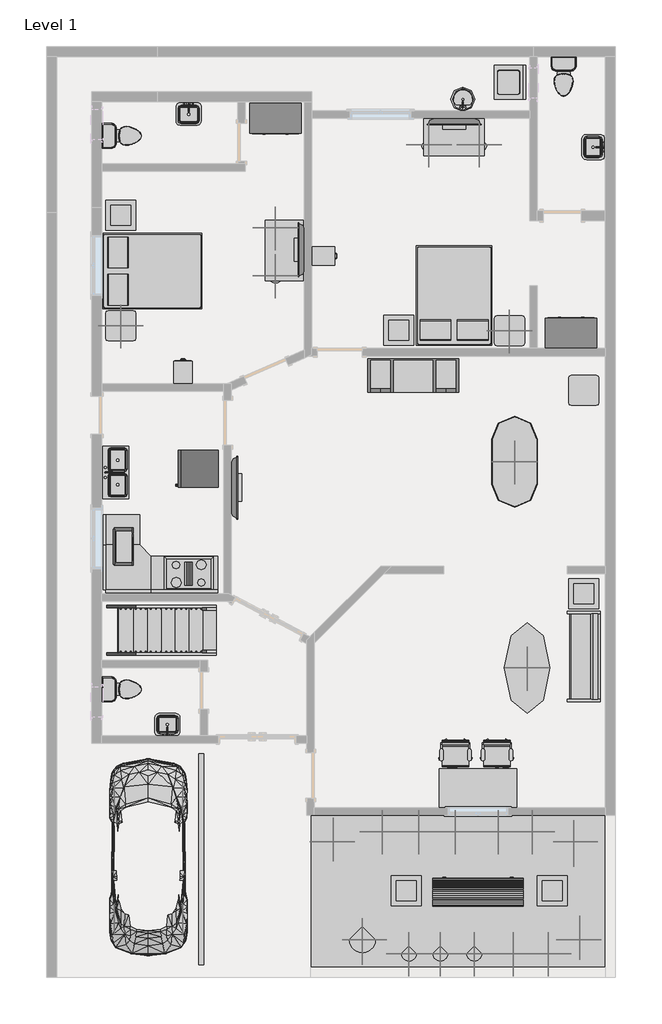
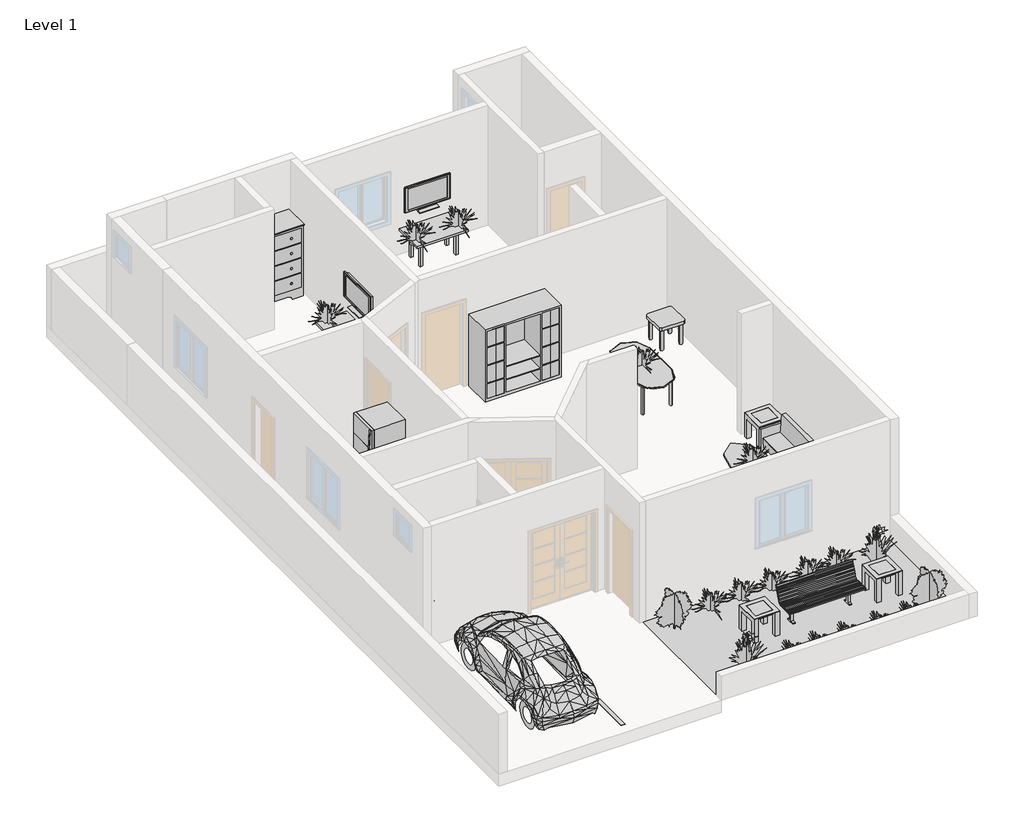
# One storey, part 2 of 2: 27 furniture elements, 23 geographic elements, 12 flow terminals, 7 proxies, 2 members, 2 railings, 1 stair flight.
# Revit data of these elements (continued)
# Type "RPC Plant - Tropical : Jungle Flame - 3'" (continued)
#   built-in parameter 1005198 = "{2, 15},{39, RPC-16-FUVJ-JWG0-MWGK-8000-ST1L-LVER-AU},{1, 0},{1, 0},{2, 13},{1, 8},{5, Color},{1, 0},{1, 0},{3, 0.8},{3, 0.8},{3, 0.8},{1, 8},{7, BBoxMin},{1, 0},{1, 0},{1, 0},{1, 0},{1, 0},{1, 8},{7, BBoxMax},{1, 0},{1, 0},{1, 0},{1, 0},{1, 0},{2, 11},{9, RPCTypeId},{1, 0},{1, 0},{39, RPC-16-FUVJ-JWG0-MWGK-8000-ST1L-LVER-AU},{1, 6},{14, RPCPlantHeight},{1, 0},{1, 0},{1, 3},{2, 11},{7, keyword},{1, 0},{1, 0},{35, :RPCs:Shrubs [General]:Geometry:RPC},{2, 11},{8, category},{1, 0},{1, 0},{16, Shrubs [General]},{2, 11},{12, LocalizedUID},{1, 0},{1, 0},{12, Jungle Flame},{2, 14},{6, Height},{1, 0},{1, 0},{1, 3},{1, 2},{16, Cast Reflections},{1, 0},{1, 0},{1, 0},{1, 2},{12, Cast Shadows},{1, 0},{1, 0},{1, 1},{1, 2},{9, Lock View},{1, 0},{1, 0},{1, 0},{1, 4},{5, ViewC},{1, 0},{1, 0},{1, 0},{21, assetlibrary_base.fbx},{1, 5},"
#   built-in parameter 1005195 = "RPC-16-FUVJ-JWG0-MWGK-8000-ST1L-LVER-AU"
#   Type Comments = "Jungle Flame"
#   Assembly Code = "G2050500"
#   Height = 3' - 0"
#   Default Elevation = 0
# Type "Handrail - Rectangular"
#   Assembly Code = "C2010400"
#   built-in parameter 1008612 = 0.0416667 (stored number, unit not read)
#   built-in parameter 1008611 = 0.0416667 (stored number, unit not read)
#   built-in parameter 1008609 = 0.333333 (stored number, unit not read)
#   built-in parameter 1008604 = 0.166667 (stored number, unit not read)
#   built-in parameter 1008603 = 0.166667 (stored number, unit not read)
#   Railing Height = 3' - 0"
#   built-in parameter 1008630 = 2
#   built-in parameter 1008610 = 2
#   built-in parameter 1008618 = Baluster - Square : 3/4"
# Element 1 (IfcBuildingElementProxy)
#   Material = Plant
#   Phase Created = New Construction
# Element 2 (IfcBuildingElementProxy, "Cook Top-4 Unit : 36\" x 20\"")
#   Phase Created = New Construction
#   Materials on its faces: "Steel, Chrome Plated", "Steel, Polished"
# Element 3 (IfcBuildingElementProxy, "Microwave : 30\" x 16\" x 18\"")
#   Phase Created = New Construction
#   Materials on its faces: "Laminate, Linen, Matte", "Glass"
# Element 4 (IfcBuildingElementProxy, "Parking Space : 9' x 18' - 90 deg")
#   Phase Created = New Construction
#   Materials on its faces: "Parking Stripe"
# Element 5 (IfcBuildingElementProxy, "RPC Beetle : RPC Beetle")
#   Phase Created = New Construction
# Element 6 (IfcBuildingElementProxy, "Refrigerator : 30\" x 32\" RH")
#   Phase Created = New Construction
#   Materials on its faces: "Steel, Paint Finish, Ivory, Glossy", "Steel, Chrome Plated"
# Element 7 (IfcBuildingElementProxy, "Washer : 27\" x 25\" x 35\"")
#   Phase Created = New Construction
#   Materials on its faces: "Steel, Paint Finish, Ivory, Matte"
# Element 8 (IfcFlowTerminal, "Floor Drain - Round : 5\" Strainer - 2\" Drain")
#   Mark = "3"
#   Phase Created = New Construction
# Element 9 (IfcFlowTerminal, "Floor Drain - Round : 5\" Strainer - 2\" Drain")
#   Mark = "7"
#   Phase Created = New Construction
# Element 10 (IfcFlowTerminal, "Floor Drain - Round : 5\" Strainer - 2\" Drain")
#   Mark = "14"
#   Phase Created = New Construction
# Element 11 (IfcFlowTerminal, "Floor Drain - Round : 5\" Strainer - 2\" Drain")
#   Mark = "16"
#   Phase Created = New Construction
# Element 12 (IfcFlowTerminal, "Sink Kitchen-Double : 42\" x 21\"")
#   Mark = "11"
#   Phase Created = New Construction
#   Materials on its faces: "Steel, Polished"
# Element 13 (IfcFlowTerminal, "Sink Vanity-Round : 19\" x 19\"")
#   Mark = "15"
#   Phase Created = New Construction
#   Materials on its faces: "Porcelain, Linen", "Steel, Polished"
# Element 14 (IfcFlowTerminal, "Sink Vanity-Square : 20\" x 18\"")
#   Mark = "4"
#   Phase Created = New Construction
#   Materials on its faces: "Porcelain, Linen", "Steel, Polished"
# Element 15 (IfcFlowTerminal, "Sink Vanity-Square : 20\" x 18\"")
#   Mark = "8"
#   Phase Created = New Construction
#   Materials on its faces: "Porcelain, Linen", "Steel, Polished"
# Element 16 (IfcFlowTerminal, "Sink Vanity-Square : 20\" x 18\"")
#   Mark = "13"
#   Phase Created = New Construction
#   Materials on its faces: "Porcelain, Linen", "Steel, Polished"
# Element 17 (IfcFlowTerminal, "Toilet-Domestic-3D : Toilet-Domestic-3D")
#   Mark = "6"
#   Phase Created = New Construction
#   Materials on its faces: "Porcelain, Linen", "Laminate, Linen, Matte"
# Element 18 (IfcFlowTerminal, "Toilet-Domestic-3D : Toilet-Domestic-3D")
#   Mark = "10"
#   Phase Created = New Construction
#   Materials on its faces: "Porcelain, Linen", "Laminate, Linen, Matte"
# Element 19 (IfcFlowTerminal, "Toilet-Domestic-3D : Toilet-Domestic-3D")
#   Mark = "12"
#   Phase Created = New Construction
#   Materials on its faces: "Porcelain, Linen", "Laminate, Linen, Matte"
# Elements 20, 21 (IfcFurniture, "Bed-Box : Queen 60\" x 79\"")
#   Phase Created = New Construction
#   Materials on its faces: "Birch", "Sash"
# Elements 22, 23 (IfcFurniture, "Cabinet-File 2 Drawer : 15\" x 18\"")
#   Phase Created = New Construction
#   Materials on its faces: "Steel, Chrome Plated", "Steel, Paint Finish, Ivory, Glossy"
# Elements 24, 25 (IfcFurniture, "Chair-Task Arms : Chair-Task Arms")
#   Phase Created = New Construction
#   Materials on its faces: "Plastic, Opaque Black", "Textile - Slate Blue"
# Element 26 (IfcFurniture, "Desk : 60\" x 30\" Student")
#   Phase Created = New Construction
#   Materials on its faces: "Steel, Chrome Plated", "Laminate, Ivory, Matte", "Cherry"
# Elements 27, 28 (IfcFurniture, "Dresser : 48\" x 72\" x 24\"")
#   Phase Created = New Construction
#   Materials on its faces: "Laminate, Ivory, Matte", "Cherry", "Wood"
# Element 29 (IfcFurniture, "Entertainment Center : 72\" x 72\" x 24\"")
#   Phase Created = New Construction
#   Materials on its faces: "Wood - Teak", "Steel, Chrome Plated", "Glass - Clear, Grey"
# Element 30 (IfcFurniture, "Sofa : 72\"")
#   Phase Created = New Construction
#   Materials on its faces: "Cherry", "Linen, Beige"
# Elements 31, 32 (IfcFurniture, "TV - Flat Screen : 42\"")
#   Stand = yes
#   Phase Created = New Construction
#   Materials on its faces: "TV - Black", "TV - Glass", "TV - Screen"
# Element 33 (IfcFurniture, "TV - Flat Screen : 50\"")
#   Stand = yes
#   Phase Created = New Construction
#   Materials on its faces: "TV - Black", "TV - Glass", "TV - Screen"
# Elements 34, 35, 36, 37, 38 (IfcFurniture, "Table-Coffee : 24\" x 24\" x 24\"")
#   Phase Created = New Construction
#   Materials on its faces: "Glass - Clear, Grey"
# Element 39 (IfcFurniture, "Table-Dining Oval : 36\" x 72\"")
#   Phase Created = New Construction
#   Materials on its faces: "Steel, Chrome Plated", "Glass - Clear, Grey"
# Element 40 (IfcFurniture, "Table-Ellipse : 72\" x 36\"")
#   Phase Created = New Construction
#   Materials on its faces: "Birch", "Plywood, Sheathing"
# Elements 41, 42, 43 (IfcFurniture, "Table-End : 24\" x 24\"")
#   Phase Created = New Construction
#   Materials on its faces: "Laminate, Ivory, Matte", "Birch"
# Elements 44, 45 (IfcFurniture, "Table-Rectangular : 72\" x 30\"")
#   Phase Created = New Construction
#   Materials on its faces: "Birch"
# Element 46 (IfcFurniture, "Work Station Cubicle : 96\" x 96\"")
#   Phase Created = New Construction
#   Materials on its faces: "Textile - Light Gray", "Laminate, Ivory, Matte"
# Element 47 (IfcGeographicElement, "Park Bench : 72\"")
#   Phase Created = New Construction
#   Materials on its faces: "Wood - Teak", "Steel, Paint Finish, Dark Gray, Matte"
# Elements 48, 49 (IfcGeographicElement, "RPC Plant - Tropical")
#   Phase Created = New Construction
# Elements 50, 51, 52, 53, 54, 55, 56, 57, 58, 59, 60, 61, 62, 63, 64, 65, 66, 67 (IfcGeographicElement, "RPC Plant - Tropical : Agave - 1.5'")
#   Phase Created = New Construction
# Elements 68, 69 (IfcGeographicElement, "RPC Plant - Tropical : Jungle Flame - 3'")
#   Phase Created = New Construction
# Elements 70, 71 (IfcMember, "Stringer - 2\" Width")
#   Phase Created = New Construction
# Elements 72, 73 (IfcRailing, "Handrail - Rectangular")
#   Phase Created = New Construction
# Element 74 (IfcStairFlight, "2\" Tread 1\" Nosing 1/4\" Riser")
#   Phase Created = New Construction
# Materials
#   "Steel, Chrome Plated": class "Metal", colour RGB 17 17 17, transparency 0, Description = "Chromiuim plated steel", Cost = 0
#   "Steel, Polished": class "Metal", colour RGB 57 57 57, transparency 0, Description = "Polished steel", Cost = 0
#   "Laminate, Linen, Matte": class "Plastic", colour RGB 249 239 230, transparency 0, Description = "Plastic Laminate - Linen, Matte", Cost = 0
#   "Steel, Paint Finish, Ivory, Glossy": class "Metal", colour RGB 247 247 239, transparency 0, Description = "Steel, paint finish, ivory, glossy", Cost = 0
#   "Steel, Paint Finish, Ivory, Matte": class "Metal", colour RGB 247 247 239, transparency 0, Description = "Steel, paint finish, ivory, matte", Cost = 0
#   "Porcelain, Linen": class "Ceramic", colour RGB 249 239 230, transparency 0, Description = "Porcelain, linen", Cost = 0
#   "Birch": class "Wood", colour RGB 210 159 95, transparency 0, Description = "Betula Alleghaniensis", Cost = 0
#   "Sash": class "Wood", colour RGB 224 178 126, transparency 0
#   "Plastic, Opaque Black": class "Plastic", colour RGB 0 0 0, transparency 0.7, Description = "Plastic, generic, opaque black", Cost = 0
#   "Textile - Slate Blue": class "Fabric", colour RGB 98 102 118, transparency 0
#   "Laminate, Ivory, Matte": class "Plastic", colour RGB 247 247 239, transparency 0, Description = "Plastic Laminate - Ivory, Matte", Cost = 0
#   "Cherry": class "Wood", colour RGB 226 177 128, transparency 0, Description = "Prunus Serotina", Cost = 0
#   "Wood": class "Wood", colour RGB 0 0 0, transparency 0, Description = "Generic wood", Cost = 0
#   "Wood - Teak": class "Wood", colour RGB 145 112 90, transparency 0
#   "Linen, Beige": class "Textile", colour RGB 249 239 230, transparency 0, Description = "Linen, beige", Cost = 0
#   "Glass - Clear, Grey": class "Glass", colour RGB 252 255 255, transparency 0.64
#   "Plywood, Sheathing": class "Wood", colour RGB 212 179 113, transparency 0, Description = "Plywood, sheathing grade", Cost = 0
#   "Textile - Light Gray": class "Fabric", colour RGB 204 204 204, transparency 0
#   "Steel, Paint Finish, Dark Gray, Matte": class "Metal", colour RGB 98 98 98, transparency 0, Description = "Steel, paint finish, dark gray, matte", Cost = 0
#   "Plant": class "Generic", colour RGB 0 0 0, transparency 0, Description = "physical material", Cost = 0
#   "Glass": class "Glass", colour RGB 0 128 192, transparency 0.75, Description = "Soda Lime Glass", Cost = 0
#   "Parking Stripe": class "Paint", colour RGB 250 250 91, transparency 0
#   "TV - Black": colour RGB 49 49 49, transparency 0
#   "TV - Glass": colour RGB 157 157 157, transparency 0.9
#   "TV - Screen": colour RGB 0 0 0, transparency 0
